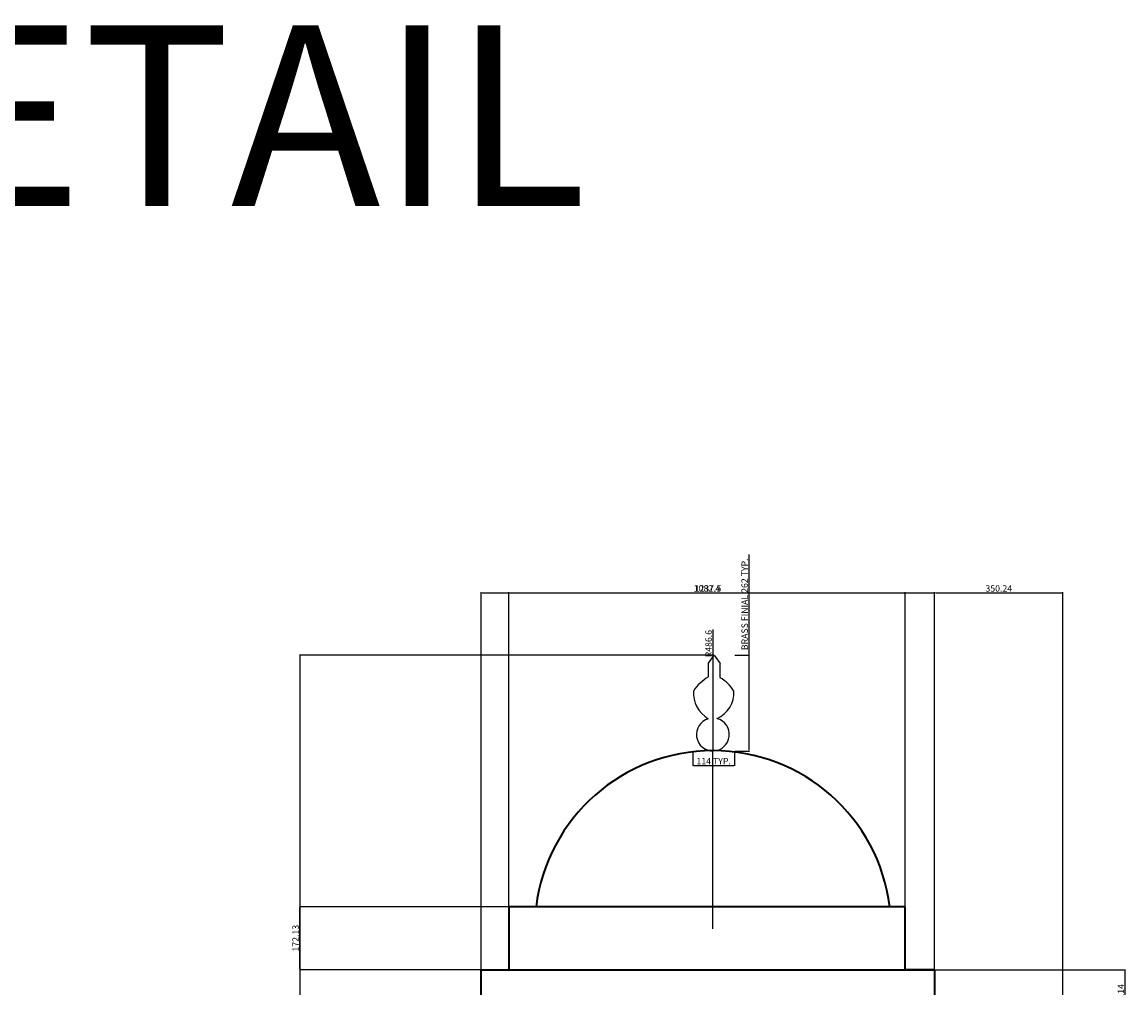
# Model space of a CAD drawing. Units: millimetres. Extents: x 498 to 8860, y -426 to 8717.
# Tile 9 of 9: x 4247 to 7260, y 6081 to 8717. Entities that reach past the tile are written whole.
import ezdxf

# ---------------------------------------------------------------- set-up
doc = ezdxf.new("R2010")
doc.units = ezdxf.units.MM
for name, color, linetype, lineweight in [('A-ANNO-DIMS', 2, 'Continuous', 18), ('A-ANNO-TEXT', 3, 'Continuous', 18), ('A-DETL', 7, 'Continuous', 25), ('A-ELEV', 7, 'Continuous', 35)]:
    doc.layers.add(name, color=color, linetype=linetype, lineweight=lineweight)
doc.styles.get("Standard").update_dxf_attribs({"font": 'arial.ttf'})
doc.dimstyles.new('ISO-25', dxfattribs={"dimtxt": 17.5, "dimasz": 2.5, "dimexe": 1.25, "dimexo": 0.625, "dimtad": 1, "dimdec": 0, "dimtxsty": 'Standard', "dimcen": 2.5, "dimadec": 0, "dimazin": 0, "dimtfac": 1, "dimtdec": 0, "dimtmove": 0, "dimatfit": 3, "dimfxl": 1, "dimarcsym": 0})

# ---------------------------------------------------------------- blocks, each defined once
blk = doc.blocks.new('FINIAL-BRASS')
for p, q in [((41.3, 239), (57, 261.6)), ((57, 261.6), (73.3, 238.5)), ((41.3, 202), (41.3, 239)), ((73.3, 199.9), (73.3, 238.5))]:
    blk.add_line(p, q)
for centre, radius, start, end in [((108.5, 89), 131.5, 120.7656, 145.5289), ((18.2, 106.2), 108.7, 31.7357, 59.5088), ((81.5, 158.5), 81.5, 176.5528, 239.9655), ((34.6, 158.5), 76.2, 293.2182, 3.7332), ((53.5, 44.9), 44.9, 106.5437, 75.6662)]:
    blk.add_arc(centre, radius, start, end)
blk = doc.blocks.new('*D39')
at = {"layer": 'A-ANNO-DIMS', "color": 0, "lineweight": -2, "transparency": 16777216}
for p, q in [((6231.2, 6989.3), (6231.2, 7263.6)), ((6192.6, 6989.3), (6232.5, 6989.3)), ((6231.2, 6729.8), (6231.2, 6986.8)), ((6192.6, 6727.3), (6232.5, 6727.3))]:
    blk.add_line(p, q, dxfattribs=at)
at = {"layer": 'A-ANNO-DIMS', "color": 0, "transparency": 16777216}
for points in [[(6230.8, 6986.8), (6231.7, 6986.8), (6231.2, 6989.3)], [(6230.8, 6729.8), (6231.7, 6729.8), (6231.2, 6727.3)]]:
    blk.add_solid(points, dxfattribs=at)
at = {"layer": 'Defpoints', "color": 0, "transparency": 16777216}
for p in [(6191.9, 6989.3), (6231.2, 6989.3), (6191.9, 6727.3)]:
    blk.add_point(p, dxfattribs=at)
at = {"layer": 'A-ANNO-DIMS', "color": 0, "transparency": 16777216, "insert": (6221.6, 7127.7), "char_height": 17.5, "attachment_point": 5, "rotation": 90}
blk.add_mtext('BRASS FINIAL 262 TYP.', dxfattribs=at)
blk = doc.blocks.new('*D40')
at = {"layer": 'A-ANNO-DIMS', "color": 0, "lineweight": -2, "transparency": 16777216}
for p, q in [((6077.5, 6726.6), (6077.5, 6686.7)), ((6191.9, 6726.6), (6191.9, 6686.7)), ((6080, 6688), (6189.4, 6688))]:
    blk.add_line(p, q, dxfattribs=at)
at = {"layer": 'A-ANNO-DIMS', "color": 0, "transparency": 16777216}
for points in [[(6080, 6688.4), (6080, 6687.6), (6077.5, 6688)], [(6189.4, 6688.4), (6189.4, 6687.6), (6191.9, 6688)]]:
    blk.add_solid(points, dxfattribs=at)
at = {"layer": 'Defpoints', "color": 0, "transparency": 16777216}
for p in [(6077.5, 6727.3), (6191.9, 6727.3), (6191.9, 6688)]:
    blk.add_point(p, dxfattribs=at)
at = {"layer": 'A-ANNO-DIMS', "color": 0, "transparency": 16777216, "insert": (6134.7, 6697.4), "char_height": 17.5, "attachment_point": 5}
blk.add_mtext('114 TYP.', dxfattribs=at)
blk = doc.blocks.new('*D53')
at = {"layer": 'A-ANNO-DIMS', "color": 0, "lineweight": -2, "transparency": 16777216}
for p, q in [((6135.6, 6989.3), (5004.1, 6989.3)), ((5005.3, 6986.8), (5005.3, 4249.1)), ((5199.1, 4246.6), (5004.1, 4246.6))]:
    blk.add_line(p, q, dxfattribs=at)
at = {"layer": 'A-ANNO-DIMS', "color": 0, "transparency": 16777216}
for points in [[(5004.9, 6986.8), (5005.8, 6986.8), (5005.3, 6989.3)], [(5004.9, 4249.1), (5005.8, 4249.1), (5005.3, 4246.6)]]:
    blk.add_solid(points, dxfattribs=at)
at = {"layer": 'Defpoints', "color": 0, "transparency": 16777216}
for p in [(6136.2, 6989.3), (5005.3, 4246.6), (5199.7, 4246.6)]:
    blk.add_point(p, dxfattribs=at)
at = {"layer": 'A-ANNO-DIMS', "color": 0, "transparency": 16777216, "insert": (4995.9, 5617.9), "char_height": 17.5, "attachment_point": 5, "rotation": 90}
blk.add_mtext('2742.7', dxfattribs=at)
blk = doc.blocks.new('*D58')
at = {"layer": 'A-ANNO-DIMS', "color": 0, "lineweight": -2, "transparency": 16777216}
for p, q in [((6737.8, 5980), (6737.8, 7160.5)), ((6740.3, 7159.3), (7085.6, 7159.3)), ((7088.1, 5820.9), (7088.1, 7160.5))]:
    blk.add_line(p, q, dxfattribs=at)
at = {"layer": 'A-ANNO-DIMS', "color": 0, "transparency": 16777216}
for points in [[(6740.3, 7159.7), (6740.3, 7158.9), (6737.8, 7159.3)], [(7085.6, 7159.7), (7085.6, 7158.9), (7088.1, 7159.3)]]:
    blk.add_solid(points, dxfattribs=at)
at = {"layer": 'Defpoints', "color": 0, "transparency": 16777216}
for p in [(7088.1, 7159.3), (6737.8, 5979.4), (7088.1, 5820.3)]:
    blk.add_point(p, dxfattribs=at)
at = {"layer": 'A-ANNO-DIMS', "color": 0, "transparency": 16777216, "insert": (6913, 7168.8), "char_height": 17.5, "attachment_point": 5}
blk.add_mtext('350.24', dxfattribs=at)
blk = doc.blocks.new('*D59')
at = {"layer": 'A-ANNO-DIMS', "color": 0, "lineweight": -2, "transparency": 16777216}
for p, q in [((6738.5, 6130.5), (7259.3, 6130.5)), ((7258.1, 5981.9), (7258.1, 6128)), ((6738.5, 5979.4), (7259.3, 5979.4))]:
    blk.add_line(p, q, dxfattribs=at)
at = {"layer": 'A-ANNO-DIMS', "color": 0, "transparency": 16777216}
for points in [[(7257.7, 6128), (7258.5, 6128), (7258.1, 6130.5)], [(7257.7, 5981.9), (7258.5, 5981.9), (7258.1, 5979.4)]]:
    blk.add_solid(points, dxfattribs=at)
at = {"layer": 'Defpoints', "color": 0, "transparency": 16777216}
for p in [(6737.8, 6130.5), (7258.1, 6130.5), (6737.8, 5979.4)]:
    blk.add_point(p, dxfattribs=at)
at = {"layer": 'A-ANNO-DIMS', "color": 0, "transparency": 16777216, "insert": (7248.5, 6054.9), "char_height": 17.5, "attachment_point": 5, "rotation": 90}
blk.add_mtext('151.14', dxfattribs=at)
blk = doc.blocks.new('*D60')
at = {"layer": 'A-ANNO-DIMS', "color": 0, "lineweight": -2, "transparency": 16777216}
for p, q in [((5500.4, 6131.1), (5500.4, 7160.5)), ((5502.9, 7159.3), (6735.3, 7159.3)), ((6737.8, 6131.1), (6737.8, 7160.5))]:
    blk.add_line(p, q, dxfattribs=at)
at = {"layer": 'A-ANNO-DIMS', "color": 0, "transparency": 16777216}
for points in [[(5502.9, 7159.7), (5502.9, 7158.9), (5500.4, 7159.3)], [(6735.3, 7159.7), (6735.3, 7158.9), (6737.8, 7159.3)]]:
    blk.add_solid(points, dxfattribs=at)
at = {"layer": 'Defpoints', "color": 0, "transparency": 16777216}
for p in [(6737.8, 7159.3), (5500.4, 6130.5), (6737.8, 6130.5)]:
    blk.add_point(p, dxfattribs=at)
at = {"layer": 'A-ANNO-DIMS', "color": 0, "transparency": 16777216, "insert": (6119.1, 7168.8), "char_height": 17.5, "attachment_point": 5}
blk.add_mtext('1237.5', dxfattribs=at)
blk = doc.blocks.new('*D61')
at = {"layer": 'A-ANNO-DIMS', "color": 0, "lineweight": -2, "transparency": 16777216}
for p, q in [((5574.8, 6302.6), (5004.1, 6302.6)), ((5005.3, 6133), (5005.3, 6300.1)), ((5574.8, 6130.5), (5004.1, 6130.5))]:
    blk.add_line(p, q, dxfattribs=at)
at = {"layer": 'A-ANNO-DIMS', "color": 0, "transparency": 16777216}
for points in [[(5004.9, 6300.1), (5005.8, 6300.1), (5005.3, 6302.6)], [(5004.9, 6133), (5005.8, 6133), (5005.3, 6130.5)]]:
    blk.add_solid(points, dxfattribs=at)
at = {"layer": 'Defpoints', "color": 0, "transparency": 16777216}
for p in [(5005.3, 6302.6), (5575.4, 6302.6), (5575.4, 6130.5)]:
    blk.add_point(p, dxfattribs=at)
at = {"layer": 'A-ANNO-DIMS', "color": 0, "transparency": 16777216, "insert": (4995.8, 6216.6), "char_height": 17.5, "attachment_point": 5, "rotation": 90}
blk.add_mtext('172.13', dxfattribs=at)
blk = doc.blocks.new('*D62')
at = {"layer": 'A-ANNO-DIMS', "color": 0, "lineweight": -2, "transparency": 16777216}
for p, q in [((5575.4, 6303.3), (5575.4, 7160.5)), ((5577.9, 7159.3), (6655.3, 7159.3)), ((6657.8, 6303.3), (6657.8, 7160.5))]:
    blk.add_line(p, q, dxfattribs=at)
at = {"layer": 'A-ANNO-DIMS', "color": 0, "transparency": 16777216}
for points in [[(5577.9, 7159.7), (5577.9, 7158.9), (5575.4, 7159.3)], [(6655.3, 7159.7), (6655.3, 7158.9), (6657.8, 7159.3)]]:
    blk.add_solid(points, dxfattribs=at)
at = {"layer": 'Defpoints', "color": 0, "transparency": 16777216}
for p in [(6657.8, 7159.3), (5575.4, 6302.6), (6657.8, 6302.6)]:
    blk.add_point(p, dxfattribs=at)
at = {"layer": 'A-ANNO-DIMS', "color": 0, "transparency": 16777216, "insert": (6116.6, 7168.8), "char_height": 17.5, "attachment_point": 5}
blk.add_mtext('1082.4', dxfattribs=at)
blk = doc.blocks.new('*D80')
at = {"layer": 'A-ANNO-DIMS', "color": 0, "lineweight": -2, "transparency": 16777216}
for p, q in [((6132.7, 7058.9), (6132.7, 6730.9)), ((6132.7, 6241.8), (6132.7, 6728.4))]:
    blk.add_line(p, q, dxfattribs=at)
at = {"layer": 'A-ANNO-DIMS', "color": 0, "transparency": 16777216}
blk.add_solid([(6132.3, 6730.9), (6133.1, 6730.9), (6132.7, 6728.4)], dxfattribs=at)
at = {"layer": 'Defpoints', "color": 0, "transparency": 16777216}
for p in [(6132.7, 6728.4), (6132.7, 6241.8)]:
    blk.add_point(p, dxfattribs=at)
at = {"layer": 'A-ANNO-DIMS', "color": 0, "transparency": 16777216, "insert": (6123.1, 7020.4), "char_height": 17.5, "attachment_point": 5, "rotation": 89.9993}
blk.add_mtext('R486.6', dxfattribs=at)

msp = doc.modelspace()

# ---------------------------------------------------------------- linework, layer by layer
at = {"layer": 'A-ELEV'}
for p, q in [((6657.845, 6302.629), (5575.425, 6302.629)), ((5575.425, 6302.629), (5575.425, 6130.498)), ((6657.845, 6130.498), (6657.845, 6302.629)), ((6737.845, 6130.498), (6657.845, 6130.498))]:
    msp.add_line(p, q, dxfattribs=at)
msp.add_lwpolyline([(5500.377, 6130.498), (6737.845, 6130.498), (6737.845, 5979.353), (5500.377, 5979.353)], close=True, dxfattribs=at)
msp.add_arc((6132.694, 6241.794), 486.622, 7.181616, 172.818384, dxfattribs=at)

# ---------------------------------------------------------------- block references
at = {"layer": 'A-DETL'}
msp.add_blockref('FINIAL-BRASS', (6079.186, 6727.704), dxfattribs=at)

# ---------------------------------------------------------------- texts
at = {"layer": 'A-ANNO-TEXT'}
msp.add_text('CHATTRI DETAIL', height=493.33964, dxfattribs=at).set_placement((643.54, 8214.558))

# ---------------------------------------------------------------- dimensions: what is measured, and where the dimension line sits
at = {"layer": 'A-ANNO-DIMS'}
dim = msp.add_linear_dim(base=(6231.239, 6989.279), p1=(6191.938, 6727.271), p2=(6191.938, 6989.279), angle=90, text='BRASS FINIAL <> TYP.', dimstyle='ISO-25', override={"dimdec": 0, "dimrnd": 0, "dimzin": 0, "dimlunit": 2}, dxfattribs=at)
dim.commit()
dim.dimension.update_dxf_attribs({"geometry": '*D39', "text_midpoint": (6221.565, 7127.677)})
for base, p1, p2, override, picture, middle in [((6737.845, 7159.279), (5500.377, 6130.498), (6737.845, 6130.498), {"dimdec": 1, "dimlfac": 1, "dimrnd": 0, "dimzin": 0, "dimdsep": 46, "dimlunit": 2}, '*D60', (6119.111, 7168.845)), ((6657.845, 7159.279), (5575.425, 6302.629), (6657.845, 6302.629), {"dimdec": 1, "dimlfac": 1, "dimrnd": 0, "dimzin": 0, "dimdsep": 46, "dimlunit": 2}, '*D62', (6116.635, 7168.839)), ((7088.089, 7159.279), (6737.845, 5979.353), (7088.089, 5820.26), {"dimdec": 2, "dimlfac": 1, "dimrnd": 0, "dimzin": 0, "dimdsep": 46, "dimlunit": 2}, '*D58', (6912.967, 7168.845))]:
    dim = msp.add_linear_dim(base=base, p1=p1, p2=p2, dimstyle='ISO-25', override=override, dxfattribs=at)
    dim.commit()
    dim.dimension.update_dxf_attribs({"geometry": picture, "text_midpoint": middle})
dim = msp.add_radius_dim(center=(6132.694, 6241.794), mpoint=(6132.7, 6728.416), dimstyle='ISO-25', override={"dimdec": 1, "dimlfac": 1, "dimrnd": 0, "dimzin": 0, "dimdsep": 46, "dimlunit": 2}, dxfattribs=at)
dim.commit()
dim.dimension.update_dxf_attribs({"geometry": '*D80', "text_midpoint": (6132.703, 7020.388), "dimtype": 164})
for base, p1, p2, override, picture, middle in [((5005.339, 4246.61), (6136.19, 6989.279), (5199.731, 4246.61), {"dimdec": 1, "dimlfac": 1, "dimrnd": 0, "dimzin": 0, "dimdsep": 46, "dimlunit": 2}, '*D53', (4995.928, 5617.944)), ((5005.339, 6302.629), (5575.425, 6130.498), (5575.425, 6302.629), {"dimdec": 2, "dimlfac": 1, "dimrnd": 0, "dimzin": 0, "dimdsep": 46, "dimlunit": 2}, '*D61', (4995.773, 6216.563)), ((7258.0889, 6130.49787), (6737.84498, 5979.35295), (6737.84498, 6130.49787), {"dimdec": 2, "dimlfac": 1, "dimrnd": 0, "dimzin": 0, "dimdsep": 46, "dimlunit": 2}, '*D59', (7248.52888, 6054.92541))]:
    dim = msp.add_linear_dim(base=base, p1=p1, p2=p2, angle=90, dimstyle='ISO-25', override=override, dxfattribs=at)
    dim.commit()
    dim.dimension.update_dxf_attribs({"geometry": picture, "text_midpoint": middle})
dim = msp.add_linear_dim(base=(6191.938, 6687.969), p1=(6077.473, 6727.271), p2=(6191.938, 6727.271), text='<> TYP.', dimstyle='ISO-25', override={"dimdec": 0, "dimrnd": 0, "dimzin": 0, "dimlunit": 2}, dxfattribs=at)
dim.commit()
dim.dimension.update_dxf_attribs({"geometry": '*D40', "text_midpoint": (6134.705, 6697.386)})

doc.saveas('drawing.dxf')
